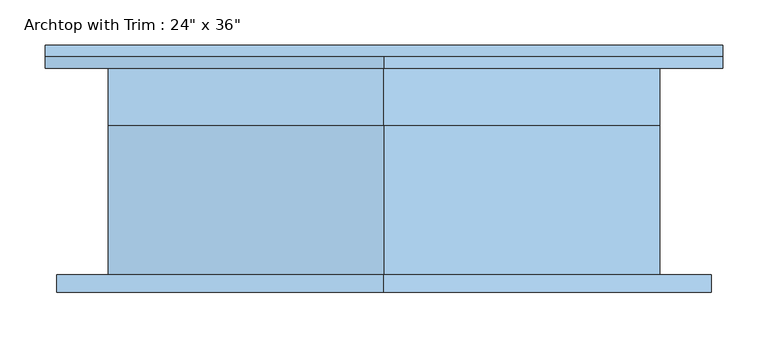
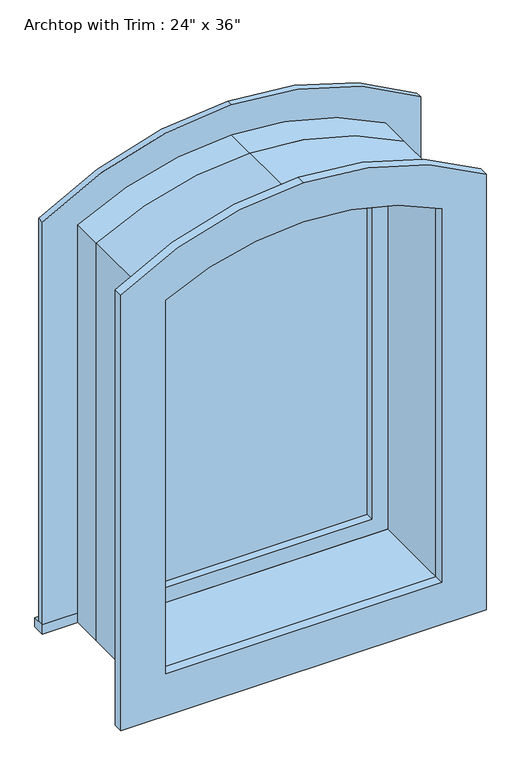
"""IFC4 building model written with IfcOpenShell, lengths in millimetres: window geometry."""

from ifc_helpers import new_model, si_unit, point, frame, frame_2d, origin, place, context, project, spatial, polyline, circle_curve, trimmed, segment, composite_curve, outline, extrude, source, transform, mapped, element, save


def window_fb83c811(model_context):
    return source(origin(), model_context, "Body", "SweptSolid", [
        extrude(outline(composite_curve([segment(polyline([(946.15, 297.730298), (1736.0135447, 297.730298)]), True, "CONTINUOUS"), segment(trimmed(circle_curve(frame_2d((1219.2, 11.980298)), 590.55), [point((1736.0135447, 297.730298))], [point((1809.75, 11.980298))], False, "CARTESIAN"), True, "CONTINUOUS"), segment(trimmed(circle_curve(frame_2d((1219.2, 11.980298)), 590.55), [point((1809.75, 11.980298))], [point((1736.0135448, -273.7697019))], False, "CARTESIAN"), True, "CONTINUOUS"), segment(polyline([(1736.0135448, -273.7697019), (946.15, -273.7697019), (946.15, 297.730298)]), True, "CONTINUOUS")], self_intersect=False), holes=[composite_curve([segment(polyline([(977.9, 253.280298), (977.9, -229.319702), (1712.6342262, -229.319702)]), True, "CONTINUOUS"), segment(trimmed(circle_curve(frame_2d((1219.2, 11.980298)), 549.275), [point((1712.6342262, -229.319702))], [point((1768.475, 11.980298))], True, "CARTESIAN"), True, "CONTINUOUS"), segment(trimmed(circle_curve(frame_2d((1219.2, 11.980298)), 549.275), [point((1768.475, 11.980298))], [point((1712.6342262, 253.280298))], True, "CARTESIAN"), True, "CONTINUOUS"), segment(polyline([(1712.6342262, 253.280298), (977.9, 253.280298)]), True, "CONTINUOUS")], self_intersect=False)]), frame((0.0, 50.8, 0.0), z_axis=(0.0, 1.0, 0.0), x_axis=(0.0, 0.0, 1.0)), (0.0, 0.0, 1.0), 44.45),
        extrude(outline(polyline([(-362.6697019, 139.7), (386.630298, 139.7), (386.630298, 114.3), (-362.6697019, 114.3), (-362.6697019, 139.7)])), frame((0.0, 0.0, 914.4), z_axis=(0.0, 0.0, 1.0), x_axis=(1.0, 0.0, 0.0)), (0.0, 0.0, 1.0), 19.05),
        extrude(outline(composite_curve([segment(polyline([(933.45, 297.7302979), (933.45, 386.630298), (1777.1420964, 386.630298)]), True, "CONTINUOUS"), segment(trimmed(circle_curve(frame_2d((1219.2, 11.980298)), 672.0580373), [point((1777.1420964, 386.630298))], [point((1891.2580373, 11.980298))], False, "CARTESIAN"), True, "CONTINUOUS"), segment(trimmed(circle_curve(frame_2d((1219.2, 11.980298)), 672.0580373), [point((1891.2580373, 11.980298))], [point((1777.1420965, -362.6697019))], False, "CARTESIAN"), True, "CONTINUOUS"), segment(polyline([(1777.1420965, -362.6697019), (933.45, -362.6697019), (933.45, -273.7697019), (1736.0135447, -273.7697019)]), True, "CONTINUOUS"), segment(trimmed(circle_curve(frame_2d((1219.2, 11.980298)), 590.55), [point((1736.0135447, -273.7697019))], [point((1809.75, 11.980298))], True, "CARTESIAN"), True, "CONTINUOUS"), segment(trimmed(circle_curve(frame_2d((1219.2, 11.980298)), 590.55), [point((1809.75, 11.980298))], [point((1736.0135448, 297.7302979))], True, "CARTESIAN"), True, "CONTINUOUS"), segment(polyline([(1736.0135448, 297.7302979), (933.45, 297.7302979)]), True, "CONTINUOUS")], self_intersect=False)), frame((0.0, 114.3, 0.0), z_axis=(0.0, 1.0, 0.0), x_axis=(0.0, 0.0, 1.0)), (0.0, 0.0, 1.0), 12.7),
        extrude(outline(composite_curve([segment(polyline([(857.25, -349.969702), (857.25, 373.9302979), (1769.9014713, 373.9302979)]), True, "CONTINUOUS"), segment(trimmed(circle_curve(frame_2d((1219.2, 11.980298)), 658.9991752), [point((1769.9014713, 373.9302979))], [point((1878.1991752, 11.980298))], False, "CARTESIAN"), True, "CONTINUOUS"), segment(trimmed(circle_curve(frame_2d((1219.2, 11.980298)), 658.9991752), [point((1878.1991752, 11.980298))], [point((1769.9014713, -349.969702))], False, "CARTESIAN"), True, "CONTINUOUS"), segment(polyline([(1769.9014713, -349.969702), (857.25, -349.969702)]), True, "CONTINUOUS")], self_intersect=False), holes=[composite_curve([segment(polyline([(946.15, -261.0697027), (1728.4684161, -261.0697027)]), True, "CONTINUOUS"), segment(trimmed(circle_curve(frame_2d((1219.2, 11.980298)), 577.85), [point((1728.4684161, -261.0697027))], [point((1797.05, 11.980298))], True, "CARTESIAN"), True, "CONTINUOUS"), segment(trimmed(circle_curve(frame_2d((1219.2000002, 11.980298)), 577.8499998), [point((1797.05, 11.980298))], [point((1728.4684161, 285.0302987))], True, "CARTESIAN"), True, "CONTINUOUS"), segment(polyline([(1728.4684161, 285.0302987), (946.15, 285.0302987), (946.15, -261.0697027)]), True, "CONTINUOUS")], self_intersect=False)]), frame((0.0, -133.35, 0.0), z_axis=(0.0, 1.0, 0.0), x_axis=(0.0, 0.0, 1.0)), (0.0, 0.0, 1.0), 19.05),
        extrude(outline(composite_curve([segment(polyline([(977.9, -229.3197017), (977.9, 253.2802981), (1712.9281367, 253.2802981)]), True, "CONTINUOUS"), segment(trimmed(circle_curve(frame_2d((1219.2, 11.9802983)), 549.5390458), [point((1712.9281367, 253.2802981))], [point((1768.7390458, 11.9802983))], False, "CARTESIAN"), True, "CONTINUOUS"), segment(trimmed(circle_curve(frame_2d((1219.2, 11.9802983)), 549.5390458), [point((1768.7390458, 11.9802983))], [point((1712.9281366, -229.3197017))], False, "CARTESIAN"), True, "CONTINUOUS"), segment(polyline([(1712.9281366, -229.3197017), (977.9, -229.3197017)]), True, "CONTINUOUS")], self_intersect=False)), frame((0.0, 66.675, 0.0), z_axis=(0.0, 1.0, 0.0), x_axis=(0.0, 0.0, 1.0)), (0.0, 0.0, 1.0), 12.7),
        extrude(outline(composite_curve([segment(polyline([(914.4, 316.780298), (1747.1290861, 316.780298)]), True, "CONTINUOUS"), segment(trimmed(circle_curve(frame_2d((1219.2, 11.980298)), 609.6), [point((1747.1290861, 316.780298))], [point((1828.8, 11.980298))], False, "CARTESIAN"), True, "CONTINUOUS"), segment(trimmed(circle_curve(frame_2d((1219.2, 11.980298)), 609.6), [point((1828.8, 11.980298))], [point((1747.1290861, -292.819702))], False, "CARTESIAN"), True, "CONTINUOUS"), segment(polyline([(1747.1290861, -292.819702), (914.4, -292.819702), (914.4, 316.780298)]), True, "CONTINUOUS")], self_intersect=False), holes=[composite_curve([segment(polyline([(946.15, 285.0302987), (946.15, -261.069702), (1732.0825062, -261.069702)]), True, "CONTINUOUS"), segment(trimmed(circle_curve(frame_2d((1219.2, 11.980298)), 581.0376646), [point((1732.0825062, -261.069702))], [point((1800.2376646, 11.980298))], True, "CARTESIAN"), True, "CONTINUOUS"), segment(trimmed(circle_curve(frame_2d((1219.2, 11.980298)), 581.0376646), [point((1800.2376646, 11.980298))], [point((1732.0825058, 285.0302987))], True, "CARTESIAN"), True, "CONTINUOUS"), segment(polyline([(1732.0825058, 285.0302987), (946.15, 285.0302987)]), True, "CONTINUOUS")], self_intersect=False)]), frame((0.0, -114.3, 0.0), z_axis=(0.0, 1.0, 0.0), x_axis=(0.0, 0.0, 1.0)), (0.0, 0.0, 1.0), 165.1),
        extrude(outline(composite_curve([segment(polyline([(914.4, -292.819702), (914.4, 316.780298), (1747.1290861, 316.780298)]), True, "CONTINUOUS"), segment(trimmed(circle_curve(frame_2d((1219.2, 11.980298)), 609.6), [point((1747.1290861, 316.780298))], [point((1828.8, 11.980298))], False, "CARTESIAN"), True, "CONTINUOUS"), segment(trimmed(circle_curve(frame_2d((1219.2, 11.980298)), 609.6), [point((1828.8, 11.980298))], [point((1747.1290861, -292.819702))], False, "CARTESIAN"), True, "CONTINUOUS"), segment(polyline([(1747.1290861, -292.819702), (914.4, -292.819702)]), True, "CONTINUOUS")], self_intersect=False), holes=[composite_curve([segment(polyline([(933.45, -273.7697019), (1738.1358634, -273.7697019)]), True, "CONTINUOUS"), segment(trimmed(circle_curve(frame_2d((1219.2, 11.980298)), 592.4082147), [point((1738.1358634, -273.7697019))], [point((1811.6082147, 11.980298))], True, "CARTESIAN"), True, "CONTINUOUS"), segment(trimmed(circle_curve(frame_2d((1219.2, 11.980298)), 592.4082147), [point((1811.6082147, 11.980298))], [point((1738.1358634, 297.730298))], True, "CARTESIAN"), True, "CONTINUOUS"), segment(polyline([(1738.1358634, 297.730298), (933.45, 297.730298), (933.45, -273.7697019)]), True, "CONTINUOUS")], self_intersect=False)]), frame((0.0, 50.8, 0.0), z_axis=(0.0, 1.0, 0.0), x_axis=(0.0, 0.0, 1.0)), (0.0, 0.0, 1.0), 63.5),
    ])


if __name__ == "__main__":
    model = new_model("IFC4")
    model_context = context("Model", 3, world=origin())
    ifc_project = project(units=[si_unit("LENGTHUNIT", "METRE", prefix="MILLI")], contexts=[model_context])
    site = spatial("IfcSite", under=ifc_project)
    building = spatial("IfcBuilding", under=site)
    placement = place(None, origin())
    window_shape = window_fb83c811(model_context)
    element("IfcWindow", 1, ObjectType="Archtop with Trim : 24\" x 36\"", at=placement, inside=building, context=model_context, shape_type="MappedRepresentation", body=[
        mapped(window_shape, transform((0.0, 0.0, 0.0), x_axis=(1.0, 0.0, 0.0), y_axis=(0.0, 1.0, 0.0), z_axis=(0.0, 0.0, 1.0))),
    ])
    save(model, "model.ifc")

# Revit data of these elements
# Type "Archtop with Trim : 24\" x 36\""
#   Type Mark = "10"
#   Construction Type Id = "GSP4R"
#   Assembly Code = "B2020100"
#   Analytic Construction = "1/8 in Pilkington single glazing"
#   Visual Light Transmittance = 0.9
#   Solar Heat Gain Coefficient = 0.78
#   Heat Transfer Coefficient (U) = 0.6496 BTU/(h·ft²·°F)
#   Height = 3' - 0"
#   Radius = 2' - 0"
#   Default Sill Height = 3' - 0"
#   Trim Projection - Ext. = 0' - 0 1/2"
#   Trim Projection - Int. = 0' - 0 3/4"
#   Trim Width - Exterior = 0' - 3 1/2"
#   Trim Width - Interior = 0' - 3 1/2"
#   Width = 2' - 0"
#   Define Thermal Properties by = 1
#   Glass Pane Material = Glass
#   Sash Material = Sash
#   Trim Exterior Material = Trim
#   Trim Interior Material = Trim
#   Wall Closure = (empty or 0)
# Element 1 (IfcWindow, "Archtop with Trim : 24\" x 36\"")
#   Materials on its faces: "Sash", "Trim", "Glass"
# Materials
#   "Glass": class "Glass", colour RGB 0 128 192, transparency 0.75, Description = "Soda Lime Glass", Cost = 0
#   "Sash": class "Wood", colour RGB 224 178 126, transparency 0
#   "Trim": class "Wood", colour RGB 224 178 126, transparency 0
